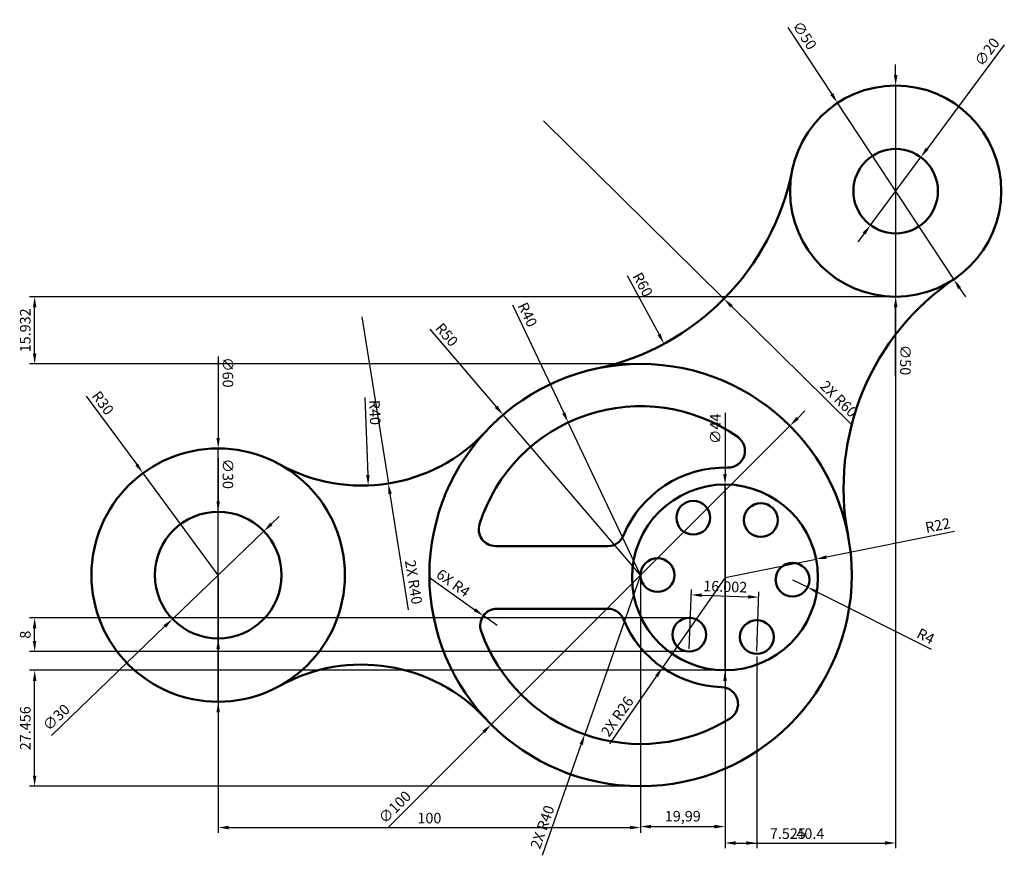
# Model space of a CAD drawing. Units: millimetres. Extents: x 2504 to 2737, y 1647 to 1845.
import ezdxf

# ---------------------------------------------------------------- set-up
doc = ezdxf.new("R2010")
doc.units = ezdxf.units.MM
doc.layers.add('M-DIMS', color=2, linetype='Continuous', lineweight=25)
doc.layers.add('M-OUTL', color=7, linetype='Continuous', lineweight=50)
doc.styles.get("Standard").update_dxf_attribs({"font": 'arial.ttf'})
doc.dimstyles.new('ISO-25', dxfattribs={"dimtxt": 2.5, "dimasz": 2.5, "dimexe": 1.25, "dimexo": 0.625, "dimtad": 1, "dimtxsty": 'Standard', "dimcen": 2.5, "dimadec": 0, "dimazin": 0, "dimtfac": 1, "dimtmove": 0, "dimatfit": 3, "dimfxl": 1, "dimarcsym": 0})

# ---------------------------------------------------------------- blocks, each defined once
blk = doc.blocks.new('*U1')
blk.add_circle((0, 0), 4)
blk = doc.blocks.new('*U2')
at = {"layer": 'M-OUTL', "color": 0, "linetype": 'ByBlock', "lineweight": -2, "transparency": 16777216}
for p, rotation in [((2663.06, 1727.21), 299.9999999999999), ((2679.05, 1726.66), 240), ((2686.57, 1712.54), 180), ((2662.11, 1699.51), 59.99999999999999), ((2678.11, 1698.96), 120)]:
    blk.add_blockref('*U1', p, dxfattribs=dict(at, rotation=rotation))
blk.add_blockref('*U1', (2654.59, 1713.63), dxfattribs=at)
blk = doc.blocks.new('*D3')
at = {"layer": 'Defpoints', "color": 0, "transparency": 16777216}
for p in [(2532.79, 1737.78), (2550.59, 1713.63)]:
    blk.add_point(p, dxfattribs=at)
at = {"layer": 'M-DIMS', "color": 0, "lineweight": -2, "transparency": 16777216}
for p, q in [((2519.37, 1755.97), (2531.3, 1739.79)), ((2550.59, 1713.63), (2532.79, 1737.78))]:
    blk.add_line(p, q, dxfattribs=at)
at = {"layer": 'M-DIMS', "color": 0, "transparency": 16777216}
blk.add_solid([(2531.64, 1740.03), (2530.97, 1739.54), (2532.79, 1737.78)], dxfattribs=at)
at = {"layer": 'M-DIMS', "color": 0, "transparency": 16777216, "insert": (2523.04, 1754.2), "char_height": 2.5, "attachment_point": 5, "rotation": 306.3975}
blk.add_mtext('R30', dxfattribs=at)
blk = doc.blocks.new('*D4')
at = {"layer": 'Defpoints', "color": 0, "transparency": 16777216}
for p in [(2584.59, 1774.82), (2586.11, 1734.85)]:
    blk.add_point(p, dxfattribs=at)
at = {"layer": 'M-DIMS', "color": 0, "lineweight": -2, "transparency": 16777216}
blk.add_line((2585.32, 1755.67), (2586.02, 1737.34), dxfattribs=at)
at = {"layer": 'M-DIMS', "color": 0, "transparency": 16777216}
blk.add_solid([(2586.44, 1737.36), (2585.6, 1737.33), (2586.11, 1734.85)], dxfattribs=at)
at = {"layer": 'M-DIMS', "color": 0, "transparency": 16777216, "insert": (2587.36, 1752.14), "char_height": 2.5, "attachment_point": 5, "rotation": 272.187}
blk.add_mtext('R40', dxfattribs=at)
blk = doc.blocks.new('*D5')
at = {"layer": 'Defpoints', "color": 0, "transparency": 16777216}
for p in [(2618.04, 1751.58), (2650.59, 1713.63)]:
    blk.add_point(p, dxfattribs=at)
at = {"layer": 'M-DIMS', "color": 0, "lineweight": -2, "transparency": 16777216}
for p, q in [((2600.66, 1771.84), (2616.41, 1753.48)), ((2650.59, 1713.63), (2618.04, 1751.58))]:
    blk.add_line(p, q, dxfattribs=at)
at = {"layer": 'M-DIMS', "color": 0, "transparency": 16777216}
blk.add_solid([(2616.73, 1753.75), (2616.09, 1753.21), (2618.04, 1751.58)], dxfattribs=at)
at = {"layer": 'M-DIMS', "color": 0, "transparency": 16777216, "insert": (2604.45, 1770.34), "char_height": 2.5, "attachment_point": 5, "rotation": 310.6195}
blk.add_mtext('R50', dxfattribs=at)
blk = doc.blocks.new('*D6')
at = {"layer": 'Defpoints', "color": 0, "transparency": 16777216}
for p in [(2633.46, 1749.78), (2650.59, 1713.63)]:
    blk.add_point(p, dxfattribs=at)
at = {"layer": 'M-DIMS', "color": 0, "lineweight": -2, "transparency": 16777216}
for p, q in [((2620.27, 1777.62), (2632.39, 1752.04)), ((2650.59, 1713.63), (2633.46, 1749.78))]:
    blk.add_line(p, q, dxfattribs=at)
at = {"layer": 'M-DIMS', "color": 0, "transparency": 16777216}
blk.add_solid([(2632.77, 1752.21), (2632.02, 1751.86), (2633.46, 1749.78)], dxfattribs=at)
at = {"layer": 'M-DIMS', "color": 0, "transparency": 16777216, "insert": (2623.54, 1775.17), "char_height": 2.5, "attachment_point": 5, "rotation": 295.3485}
blk.add_mtext('R40', dxfattribs=at)
blk = doc.blocks.new('*D7')
at = {"layer": 'Defpoints', "color": 0, "transparency": 16777216}
for p in [(2692.15, 1717.4), (2670.58, 1713.08)]:
    blk.add_point(p, dxfattribs=at)
at = {"layer": 'M-DIMS', "color": 0, "lineweight": -2, "transparency": 16777216}
for p, q in [((2724.9, 1723.96), (2694.6, 1717.9)), ((2670.58, 1713.08), (2692.15, 1717.4))]:
    blk.add_line(p, q, dxfattribs=at)
at = {"layer": 'M-DIMS', "color": 0, "transparency": 16777216}
blk.add_solid([(2694.52, 1718.3), (2694.69, 1717.49), (2692.15, 1717.4)], dxfattribs=at)
at = {"layer": 'M-DIMS', "color": 0, "transparency": 16777216, "insert": (2721, 1725.1), "char_height": 2.5, "attachment_point": 5, "rotation": 11.3281}
blk.add_mtext('R22', dxfattribs=at)
blk = doc.blocks.new('*D8')
at = {"layer": 'Defpoints', "color": 0, "transparency": 16777216}
for p in [(2686.57, 1712.54), (2690.15, 1710.74)]:
    blk.add_point(p, dxfattribs=at)
at = {"layer": 'M-DIMS', "color": 0, "lineweight": -2, "transparency": 16777216}
for p, q in [((2686.57, 1712.54), (2690.15, 1710.74)), ((2719.46, 1696.02), (2692.38, 1709.62))]:
    blk.add_line(p, q, dxfattribs=at)
at = {"layer": 'M-DIMS', "color": 0, "transparency": 16777216}
blk.add_solid([(2692.57, 1709.99), (2692.2, 1709.25), (2690.15, 1710.74)], dxfattribs=at)
at = {"layer": 'M-DIMS', "color": 0, "transparency": 16777216, "insert": (2717.95, 1698.88), "char_height": 2.5, "attachment_point": 5, "rotation": 333.3339}
blk.add_mtext('R4', dxfattribs=at)
blk = doc.blocks.new('*D9')
at = {"layer": 'Defpoints', "color": 0, "transparency": 16777216}
for p in [(2627.63, 1821.2), (2656.15, 1768.42)]:
    blk.add_point(p, dxfattribs=at)
at = {"layer": 'M-DIMS', "color": 0, "lineweight": -2, "transparency": 16777216}
blk.add_line((2647.43, 1784.55), (2654.96, 1770.62), dxfattribs=at)
at = {"layer": 'M-DIMS', "color": 0, "transparency": 16777216}
blk.add_solid([(2655.33, 1770.82), (2654.6, 1770.42), (2656.15, 1768.42)], dxfattribs=at)
at = {"layer": 'M-DIMS', "color": 0, "transparency": 16777216, "insert": (2650.82, 1782.28), "char_height": 2.5, "attachment_point": 5, "rotation": 298.3875}
blk.add_mtext('R60', dxfattribs=at)
blk = doc.blocks.new('*D10')
at = {"layer": 'Defpoints', "color": 0, "transparency": 16777216}
for p in [(2716.94, 1812.59), (2705.02, 1796.53)]:
    blk.add_point(p, dxfattribs=at)
at = {"layer": 'M-DIMS', "color": 0, "lineweight": -2, "transparency": 16777216}
for p, q in [((2736.7, 1839.2), (2718.43, 1814.6)), ((2705.02, 1796.53), (2716.94, 1812.59)), ((2703.53, 1794.52), (2702.04, 1792.52))]:
    blk.add_line(p, q, dxfattribs=at)
at = {"layer": 'M-DIMS', "color": 0, "transparency": 16777216}
for points in [[(2718.1, 1814.84), (2718.77, 1814.35), (2716.94, 1812.59)], [(2703.19, 1794.77), (2703.86, 1794.28), (2705.02, 1796.53)]]:
    blk.add_solid(points, dxfattribs=at)
at = {"layer": 'M-DIMS', "color": 0, "transparency": 16777216, "insert": (2732.87, 1837.34), "char_height": 2.5, "attachment_point": 5, "rotation": 53.4}
blk.add_mtext('∅20', dxfattribs=at)
blk = doc.blocks.new('*D11')
at = {"layer": 'Defpoints', "color": 0, "transparency": 16777216}
for p in [(2697.23, 1825.44), (2724.73, 1783.68)]:
    blk.add_point(p, dxfattribs=at)
at = {"layer": 'M-DIMS', "color": 0, "lineweight": -2, "transparency": 16777216}
for p, q in [((2685.45, 1843.33), (2695.85, 1827.53)), ((2724.73, 1783.68), (2697.23, 1825.44)), ((2726.11, 1781.59), (2727.48, 1779.51))]:
    blk.add_line(p, q, dxfattribs=at)
at = {"layer": 'M-DIMS', "color": 0, "transparency": 16777216}
for points in [[(2696.2, 1827.76), (2695.51, 1827.3), (2697.23, 1825.44)], [(2726.45, 1781.82), (2725.76, 1781.36), (2724.73, 1783.68)]]:
    blk.add_solid(points, dxfattribs=at)
at = {"layer": 'M-DIMS', "color": 0, "transparency": 16777216, "insert": (2689.17, 1841.26), "char_height": 2.5, "attachment_point": 5, "rotation": 303.3687}
blk.add_mtext('∅50', dxfattribs=at)
blk = doc.blocks.new('*D12')
at = {"layer": 'Defpoints', "color": 0, "transparency": 16777216}
for p in [(2561.4, 1724.02), (2539.78, 1703.23)]:
    blk.add_point(p, dxfattribs=at)
at = {"layer": 'M-DIMS', "color": 0, "lineweight": -2, "transparency": 16777216}
for p, q in [((2563.2, 1725.76), (2565, 1727.49)), ((2561.4, 1724.02), (2539.78, 1703.23)), ((2511.12, 1675.67), (2537.97, 1701.5))]:
    blk.add_line(p, q, dxfattribs=at)
at = {"layer": 'M-DIMS', "color": 0, "transparency": 16777216}
for points in [[(2562.91, 1726.06), (2563.49, 1725.46), (2561.4, 1724.02)], [(2537.69, 1701.8), (2538.26, 1701.2), (2539.78, 1703.23)]]:
    blk.add_solid(points, dxfattribs=at)
at = {"layer": 'M-DIMS', "color": 0, "transparency": 16777216, "insert": (2512.47, 1679.71), "char_height": 2.5, "attachment_point": 5, "rotation": 43.8787}
blk.add_mtext('∅30', dxfattribs=at)
blk = doc.blocks.new('*D13')
at = {"layer": 'Defpoints', "color": 0, "transparency": 16777216}
for p in [(2550.59, 1713.63), (2650.59, 1713.63), (2650.59, 1653.85)]:
    blk.add_point(p, dxfattribs=at)
at = {"layer": 'M-DIMS', "color": 0, "lineweight": -2, "transparency": 16777216}
for p, q in [((2550.59, 1713), (2550.59, 1652.6)), ((2650.59, 1713), (2650.59, 1652.6)), ((2553.09, 1653.85), (2648.09, 1653.85))]:
    blk.add_line(p, q, dxfattribs=at)
at = {"layer": 'M-DIMS', "color": 0, "transparency": 16777216}
for points in [[(2553.09, 1654.26), (2553.09, 1653.43), (2550.59, 1653.85)], [(2648.09, 1654.26), (2648.09, 1653.43), (2650.59, 1653.85)]]:
    blk.add_solid(points, dxfattribs=at)
at = {"layer": 'M-DIMS', "color": 0, "transparency": 16777216, "insert": (2600.59, 1655.75), "char_height": 2.5, "attachment_point": 5}
blk.add_mtext('100', dxfattribs=at)
blk = doc.blocks.new('*D14')
at = {"layer": 'Defpoints', "color": 0, "transparency": 16777216}
for p in [(2650.59, 1713.08), (2670.58, 1713.08), (2670.58, 1654.07)]:
    blk.add_point(p, dxfattribs=at)
at = {"layer": 'M-DIMS', "color": 0, "lineweight": -2, "transparency": 16777216}
for p, q in [((2650.59, 1712.46), (2650.59, 1652.82)), ((2670.58, 1712.46), (2670.58, 1652.82)), ((2653.09, 1654.07), (2668.08, 1654.07))]:
    blk.add_line(p, q, dxfattribs=at)
at = {"layer": 'M-DIMS', "color": 0, "transparency": 16777216}
for points in [[(2653.09, 1654.49), (2653.09, 1653.65), (2650.59, 1654.07)], [(2668.08, 1654.49), (2668.08, 1653.65), (2670.58, 1654.07)]]:
    blk.add_solid(points, dxfattribs=at)
at = {"layer": 'M-DIMS', "color": 0, "transparency": 16777216, "insert": (2660.58, 1656.2), "char_height": 2.5, "attachment_point": 5}
blk.add_mtext('19,99', dxfattribs=at)
blk = doc.blocks.new('*D15')
at = {"layer": 'Defpoints', "color": 0, "transparency": 16777216}
for p in [(2507.14, 1779.56), (2710.98, 1779.56), (2650.59, 1763.63)]:
    blk.add_point(p, dxfattribs=at)
at = {"layer": 'M-DIMS', "color": 0, "lineweight": -2, "transparency": 16777216}
for p, q in [((2710.35, 1779.56), (2505.89, 1779.56)), ((2507.14, 1766.13), (2507.14, 1777.06)), ((2649.96, 1763.63), (2505.89, 1763.63))]:
    blk.add_line(p, q, dxfattribs=at)
at = {"layer": 'M-DIMS', "color": 0, "transparency": 16777216}
for points in [[(2506.72, 1777.06), (2507.55, 1777.06), (2507.14, 1779.56)], [(2506.72, 1766.13), (2507.55, 1766.13), (2507.14, 1763.63)]]:
    blk.add_solid(points, dxfattribs=at)
at = {"layer": 'M-DIMS', "color": 0, "transparency": 16777216, "insert": (2505.24, 1771.59), "char_height": 2.5, "attachment_point": 5, "rotation": 90}
blk.add_mtext('15.932', dxfattribs=at)
blk = doc.blocks.new('*D16')
at = {"layer": 'Defpoints', "color": 0, "transparency": 16777216}
for p in [(2710.98, 1779.56), (2670.58, 1735.08), (2710.98, 1650.18)]:
    blk.add_point(p, dxfattribs=at)
at = {"layer": 'M-DIMS', "color": 0, "lineweight": -2, "transparency": 16777216}
for p, q in [((2710.98, 1778.93), (2710.98, 1648.93)), ((2670.58, 1734.46), (2670.58, 1648.93)), ((2673.08, 1650.18), (2708.48, 1650.18))]:
    blk.add_line(p, q, dxfattribs=at)
at = {"layer": 'M-DIMS', "color": 0, "transparency": 16777216}
for points in [[(2673.08, 1650.59), (2673.08, 1649.76), (2670.58, 1650.18)], [(2708.48, 1650.59), (2708.48, 1649.76), (2710.98, 1650.18)]]:
    blk.add_solid(points, dxfattribs=at)
at = {"layer": 'M-DIMS', "color": 0, "transparency": 16777216, "insert": (2690.78, 1652.08), "char_height": 2.5, "attachment_point": 5}
blk.add_mtext('40.4', dxfattribs=at)
blk = doc.blocks.new('*D17')
at = {"layer": 'Defpoints', "color": 0, "transparency": 16777216}
for p in [(2507.14, 1703.51), (2662.11, 1703.51), (2662.11, 1695.51)]:
    blk.add_point(p, dxfattribs=at)
at = {"layer": 'M-DIMS', "color": 0, "lineweight": -2, "transparency": 16777216}
for p, q in [((2661.49, 1703.51), (2505.89, 1703.51)), ((2507.14, 1698.01), (2507.14, 1701.01)), ((2661.49, 1695.51), (2505.89, 1695.51))]:
    blk.add_line(p, q, dxfattribs=at)
at = {"layer": 'M-DIMS', "color": 0, "transparency": 16777216}
for points in [[(2506.72, 1701.01), (2507.55, 1701.01), (2507.14, 1703.51)], [(2506.72, 1698.01), (2507.55, 1698.01), (2507.14, 1695.51)]]:
    blk.add_solid(points, dxfattribs=at)
at = {"layer": 'M-DIMS', "color": 0, "transparency": 16777216, "insert": (2505.24, 1699.51), "char_height": 2.5, "attachment_point": 5, "rotation": 90}
blk.add_mtext('8', dxfattribs=at)
blk = doc.blocks.new('*D18')
at = {"layer": 'Defpoints', "color": 0, "transparency": 16777216}
for p in [(2678.56, 1708.4), (2662.11, 1695.51), (2678.11, 1694.96)]:
    blk.add_point(p, dxfattribs=at)
at = {"layer": 'M-DIMS', "color": 0, "lineweight": -2, "transparency": 16777216}
for p, q in [((2662.13, 1696.13), (2662.61, 1710.2)), ((2665.07, 1708.86), (2676.06, 1708.49)), ((2678.13, 1695.59), (2678.61, 1709.65))]:
    blk.add_line(p, q, dxfattribs=at)
at = {"layer": 'M-DIMS', "color": 0, "transparency": 16777216}
for points in [[(2665.08, 1709.28), (2665.06, 1708.45), (2662.57, 1708.95)], [(2676.08, 1708.9), (2676.05, 1708.07), (2678.56, 1708.4)]]:
    blk.add_solid(points, dxfattribs=at)
at = {"layer": 'M-DIMS', "color": 0, "transparency": 16777216, "insert": (2670.63, 1710.58), "char_height": 2.5, "attachment_point": 5, "rotation": 358.0504}
blk.add_mtext('16.002', dxfattribs=at)
blk = doc.blocks.new('*D19')
at = {"layer": 'Defpoints', "color": 0, "transparency": 16777216}
for p in [(2507.14, 1691.08), (2670.58, 1691.08), (2650.59, 1663.63)]:
    blk.add_point(p, dxfattribs=at)
at = {"layer": 'M-DIMS', "color": 0, "lineweight": -2, "transparency": 16777216}
for p, q in [((2669.96, 1691.08), (2505.89, 1691.08)), ((2507.14, 1666.13), (2507.14, 1688.58)), ((2649.96, 1663.63), (2505.89, 1663.63))]:
    blk.add_line(p, q, dxfattribs=at)
at = {"layer": 'M-DIMS', "color": 0, "transparency": 16777216}
for points in [[(2506.72, 1688.58), (2507.55, 1688.58), (2507.14, 1691.08)], [(2506.72, 1666.13), (2507.55, 1666.13), (2507.14, 1663.63)]]:
    blk.add_solid(points, dxfattribs=at)
at = {"layer": 'M-DIMS', "color": 0, "transparency": 16777216, "insert": (2505.24, 1677.36), "char_height": 2.5, "attachment_point": 5, "rotation": 90}
blk.add_mtext('27.456', dxfattribs=at)
blk = doc.blocks.new('*D20')
at = {"layer": 'Defpoints', "color": 0, "transparency": 16777216}
for p in [(2678.11, 1694.96), (2670.58, 1691.08), (2678.11, 1650.18)]:
    blk.add_point(p, dxfattribs=at)
at = {"layer": 'M-DIMS', "color": 0, "lineweight": -2, "transparency": 16777216}
for p, q in [((2678.11, 1694.34), (2678.11, 1648.93)), ((2670.58, 1690.46), (2670.58, 1648.93)), ((2673.08, 1650.18), (2675.61, 1650.18)), ((2678.11, 1650.18), (2690.29, 1650.18))]:
    blk.add_line(p, q, dxfattribs=at)
at = {"layer": 'M-DIMS', "color": 0, "transparency": 16777216}
for points in [[(2673.08, 1650.59), (2673.08, 1649.76), (2670.58, 1650.18)], [(2675.61, 1650.59), (2675.61, 1649.76), (2678.11, 1650.18)]]:
    blk.add_solid(points, dxfattribs=at)
at = {"layer": 'M-DIMS', "color": 0, "transparency": 16777216, "insert": (2685.45, 1652.08), "char_height": 2.5, "attachment_point": 5}
blk.add_mtext('7.525', dxfattribs=at)
blk = doc.blocks.new('*D21')
at = {"layer": 'Defpoints', "color": 0, "transparency": 16777216}
for p in [(2550.59, 1743.63), (2550.59, 1683.63)]:
    blk.add_point(p, dxfattribs=at)
at = {"layer": 'M-DIMS', "color": 0, "lineweight": -2, "transparency": 16777216}
for p, q in [((2550.59, 1765.4), (2550.59, 1746.13)), ((2550.59, 1683.63), (2550.59, 1743.63)), ((2550.59, 1681.13), (2550.59, 1678.63))]:
    blk.add_line(p, q, dxfattribs=at)
at = {"layer": 'M-DIMS', "color": 0, "transparency": 16777216}
for points in [[(2551, 1746.13), (2550.17, 1746.13), (2550.59, 1743.63)], [(2551.01, 1681.13), (2550.17, 1681.13), (2550.59, 1683.63)]]:
    blk.add_solid(points, dxfattribs=at)
at = {"layer": 'M-DIMS', "color": 0, "transparency": 16777216, "insert": (2552.56, 1761.63), "char_height": 2.5, "attachment_point": 5, "rotation": 270.0006}
blk.add_mtext('∅60', dxfattribs=at)
blk = doc.blocks.new('*D22')
at = {"layer": 'Defpoints', "color": 0, "transparency": 16777216}
for p in [(2550.59, 1728.63), (2550.59, 1698.63)]:
    blk.add_point(p, dxfattribs=at)
at = {"layer": 'M-DIMS', "color": 0, "lineweight": -2, "transparency": 16777216}
for p, q in [((2550.59, 1741.4), (2550.59, 1731.13)), ((2550.59, 1698.63), (2550.59, 1728.63)), ((2550.59, 1696.13), (2550.59, 1693.63))]:
    blk.add_line(p, q, dxfattribs=at)
at = {"layer": 'M-DIMS', "color": 0, "transparency": 16777216}
for points in [[(2551, 1731.13), (2550.17, 1731.13), (2550.59, 1728.63)], [(2551.01, 1696.13), (2550.17, 1696.13), (2550.59, 1698.63)]]:
    blk.add_solid(points, dxfattribs=at)
at = {"layer": 'M-DIMS', "color": 0, "transparency": 16777216, "insert": (2552.56, 1737.63), "char_height": 2.5, "attachment_point": 5, "rotation": 270.0012}
blk.add_mtext('∅30', dxfattribs=at)
blk = doc.blocks.new('*D23')
at = {"layer": 'Defpoints', "color": 0, "transparency": 16777216}
for p in [(2685.94, 1748.98), (2615.23, 1678.27)]:
    blk.add_point(p, dxfattribs=at)
at = {"layer": 'M-DIMS', "color": 0, "lineweight": -2, "transparency": 16777216}
for p, q in [((2687.71, 1750.75), (2689.48, 1752.52)), ((2685.94, 1748.98), (2615.23, 1678.27)), ((2590.67, 1653.71), (2613.46, 1676.5))]:
    blk.add_line(p, q, dxfattribs=at)
at = {"layer": 'M-DIMS', "color": 0, "transparency": 16777216}
for points in [[(2687.42, 1751.05), (2688.01, 1750.46), (2685.94, 1748.98)], [(2613.17, 1676.8), (2613.76, 1676.21), (2615.23, 1678.27)]]:
    blk.add_solid(points, dxfattribs=at)
at = {"layer": 'M-DIMS', "color": 0, "transparency": 16777216, "insert": (2592.63, 1658.45), "char_height": 2.5, "attachment_point": 5, "rotation": 44.9996}
blk.add_mtext('∅100', dxfattribs=at)
blk = doc.blocks.new('*D24')
at = {"layer": 'Defpoints', "color": 0, "transparency": 16777216}
for p in [(2710.98, 1829.56), (2710.98, 1779.56)]:
    blk.add_point(p, dxfattribs=at)
at = {"layer": 'M-DIMS', "color": 0, "lineweight": -2, "transparency": 16777216}
for p, q in [((2710.98, 1832.06), (2710.98, 1834.56)), ((2710.98, 1829.56), (2710.98, 1779.56)), ((2710.98, 1760.79), (2710.98, 1777.06))]:
    blk.add_line(p, q, dxfattribs=at)
at = {"layer": 'M-DIMS', "color": 0, "transparency": 16777216}
for points in [[(2711.4, 1832.06), (2710.56, 1832.06), (2710.98, 1829.56)], [(2711.4, 1777.06), (2710.56, 1777.06), (2710.98, 1779.56)]]:
    blk.add_solid(points, dxfattribs=at)
at = {"layer": 'M-DIMS', "color": 0, "transparency": 16777216, "insert": (2712.95, 1764.56), "char_height": 2.5, "attachment_point": 5, "rotation": 270.0005}
blk.add_mtext('∅50', dxfattribs=at)
blk = doc.blocks.new('*D25')
at = {"layer": 'Defpoints', "color": 0, "transparency": 16777216}
for p in [(2584.59, 1774.82), (2590.88, 1735.31)]:
    blk.add_point(p, dxfattribs=at)
at = {"layer": 'M-DIMS', "color": 0, "lineweight": -2, "transparency": 16777216}
for p, q in [((2584.59, 1774.82), (2590.88, 1735.31)), ((2595.65, 1705.38), (2591.28, 1732.85))]:
    blk.add_line(p, q, dxfattribs=at)
at = {"layer": 'M-DIMS', "color": 0, "transparency": 16777216}
blk.add_solid([(2591.69, 1732.91), (2590.86, 1732.78), (2590.88, 1735.31)], dxfattribs=at)
at = {"layer": 'M-DIMS', "color": 0, "transparency": 16777216, "insert": (2596.54, 1711.91), "char_height": 2.5, "attachment_point": 5, "rotation": 279.054}
blk.add_mtext('2X R40', dxfattribs=at)
blk = doc.blocks.new('*D26')
at = {"layer": 'Defpoints', "color": 0, "transparency": 16777216}
for p in [(2650.59, 1713.63), (2637.37, 1675.88)]:
    blk.add_point(p, dxfattribs=at)
at = {"layer": 'M-DIMS', "color": 0, "lineweight": -2, "transparency": 16777216}
for p, q in [((2650.59, 1713.63), (2637.37, 1675.88)), ((2627.35, 1647.27), (2636.54, 1673.52))]:
    blk.add_line(p, q, dxfattribs=at)
at = {"layer": 'M-DIMS', "color": 0, "transparency": 16777216}
blk.add_solid([(2636.15, 1673.65), (2636.93, 1673.38), (2637.37, 1675.88)], dxfattribs=at)
at = {"layer": 'M-DIMS', "color": 0, "transparency": 16777216, "insert": (2627.64, 1653.85), "char_height": 2.5, "attachment_point": 5, "rotation": 70.6989}
blk.add_mtext('2X R40', dxfattribs=at)
blk = doc.blocks.new('*D27')
at = {"layer": 'Defpoints', "color": 0, "transparency": 16777216}
for p in [(2670.58, 1713.08), (2655.78, 1691.71)]:
    blk.add_point(p, dxfattribs=at)
at = {"layer": 'M-DIMS', "color": 0, "lineweight": -2, "transparency": 16777216}
for p, q in [((2670.58, 1713.08), (2655.78, 1691.71)), ((2643.31, 1673.68), (2654.36, 1689.65))]:
    blk.add_line(p, q, dxfattribs=at)
at = {"layer": 'M-DIMS', "color": 0, "transparency": 16777216}
blk.add_solid([(2654.02, 1689.89), (2654.7, 1689.41), (2655.78, 1691.71)], dxfattribs=at)
at = {"layer": 'M-DIMS', "color": 0, "transparency": 16777216, "insert": (2645.34, 1679.96), "char_height": 2.5, "attachment_point": 5, "rotation": 55.3063}
blk.add_mtext('2X R26', dxfattribs=at)
blk = doc.blocks.new('*D28')
at = {"layer": 'Defpoints', "color": 0, "transparency": 16777216}
for p in [(2613.37, 1703.98), (2616.63, 1701.67)]:
    blk.add_point(p, dxfattribs=at)
at = {"layer": 'M-DIMS', "color": 0, "lineweight": -2, "transparency": 16777216}
for p, q in [((2600.59, 1713.03), (2611.33, 1705.43)), ((2616.63, 1701.67), (2613.37, 1703.98))]:
    blk.add_line(p, q, dxfattribs=at)
at = {"layer": 'M-DIMS', "color": 0, "transparency": 16777216}
blk.add_solid([(2611.57, 1705.77), (2611.09, 1705.09), (2613.37, 1703.98)], dxfattribs=at)
at = {"layer": 'M-DIMS', "color": 0, "transparency": 16777216, "insert": (2606.04, 1711.5), "char_height": 2.5, "attachment_point": 5, "rotation": 324.6997}
blk.add_mtext('6X R4', dxfattribs=at)
blk = doc.blocks.new('*D29')
at = {"layer": 'Defpoints', "color": 0, "transparency": 16777216}
for p in [(2627.63, 1821.2), (2670.33, 1779.06)]:
    blk.add_point(p, dxfattribs=at)
at = {"layer": 'M-DIMS', "color": 0, "lineweight": -2, "transparency": 16777216}
for p, q in [((2627.63, 1821.2), (2670.33, 1779.06)), ((2700.45, 1749.34), (2672.11, 1777.3))]:
    blk.add_line(p, q, dxfattribs=at)
at = {"layer": 'M-DIMS', "color": 0, "transparency": 16777216}
blk.add_solid([(2672.4, 1777.6), (2671.82, 1777.01), (2670.33, 1779.06)], dxfattribs=at)
at = {"layer": 'M-DIMS', "color": 0, "transparency": 16777216, "insert": (2697.29, 1755.13), "char_height": 2.5, "attachment_point": 5, "rotation": 315.3784}
blk.add_mtext('2X R60', dxfattribs=at)
blk = doc.blocks.new('*D30')
at = {"layer": 'Defpoints', "color": 0, "transparency": 16777216}
for p in [(2670.58, 1735.08), (2670.58, 1691.08)]:
    blk.add_point(p, dxfattribs=at)
at = {"layer": 'M-DIMS', "color": 0, "lineweight": -2, "transparency": 16777216}
for p, q in [((2670.58, 1752.05), (2670.58, 1737.58)), ((2670.58, 1691.08), (2670.58, 1735.08)), ((2670.58, 1688.58), (2670.58, 1686.08))]:
    blk.add_line(p, q, dxfattribs=at)
at = {"layer": 'M-DIMS', "color": 0, "transparency": 16777216}
for points in [[(2670.16, 1737.58), (2671, 1737.58), (2670.58, 1735.08)], [(2670.16, 1688.58), (2671, 1688.58), (2670.58, 1691.08)]]:
    blk.add_solid(points, dxfattribs=at)
at = {"layer": 'M-DIMS', "color": 0, "transparency": 16777216, "insert": (2668.61, 1748.28), "char_height": 2.5, "attachment_point": 5, "rotation": 89.9997}
blk.add_mtext('∅44', dxfattribs=at)

msp = doc.modelspace()

# ---------------------------------------------------------------- linework, layer by layer
at = {"layer": 'M-OUTL'}
for p, q in [((2642.837, 1720.4971), (2616.2684, 1720.4971)), ((2642.837, 1705.6696), (2616.6324, 1705.6696))]:
    msp.add_line(p, q, dxfattribs=at)
for centre, radius in [((2710.9798, 1804.5598), 25), ((2710.9798, 1804.5598), 10), ((2650.5883, 1713.6278), 50), ((2550.5883, 1713.6278), 30), ((2670.5809, 1713.0834), 22), ((2550.5883, 1713.6278), 15)]:
    msp.add_circle(centre, radius, dxfattribs=at)
for centre, radius, start, end in [((2627.6253, 1821.2043), 60, 282.049362, 348.707517), ((2758.6502, 1734.1856), 60, 124.113141, 190.771295), ((2650.5883, 1713.6278), 40, 54.882444, 162.426663), ((2584.5883, 1774.816), 40, 240.940719, 317.166572), ((2671.2975, 1743.0748), 4, 268.63122, 54.882444), ((2670.5809, 1713.0834), 26, 88.63122, 157.637945), ((2616.2684, 1724.4971), 4, 162.426663, 270), ((2642.837, 1724.4971), 4, 270, 337.637945), ((2650.5883, 1713.6278), 40, 358.093678, 358.440234), ((2616.6324, 1701.6696), 4, 90, 199.400562), ((2642.837, 1701.6696), 4, 22.362055, 90), ((2670.5809, 1713.0834), 26, 202.362055, 268.249248), ((2650.5883, 1713.6278), 40, 199.400562, 301.998024), ((2584.5883, 1652.4395), 40, 42.833428, 119.059281), ((2669.6644, 1683.0974), 4, 301.998024, 88.249248)]:
    msp.add_arc(centre, radius, start, end, dxfattribs=at)

# ---------------------------------------------------------------- block references
msp.add_blockref('*U2', (0, 0), dxfattribs=at)

# ---------------------------------------------------------------- dimensions: what is measured, and where the dimension line sits
at = {"layer": 'M-DIMS'}
for p1, p2, override, picture, middle in [((2724.7304, 1783.6811), (2697.2291, 1825.4385), {"dimclrd": 0, "dimclre": 0, "dimclrt": 0}, '*D11', (2687.5234, 1840.1756)), ((2705.0175, 1796.5316), (2716.942, 1812.588), {"dimclrd": 0, "dimclre": 0, "dimclrt": 0}, '*D10', (2734.4544, 1836.1685)), ((2710.9795, 1829.5598), (2710.98, 1779.5598), {"dimdec": 0, "dimlfac": 1, "dimrnd": 0, "dimzin": 0, "dimdsep": 46, "dimlunit": 2}, '*D24', (2710.9801, 1764.5598)), ((2550.5886, 1683.6278), (2550.588, 1743.6278), {"dimdec": 0, "dimlfac": 1, "dimrnd": 0, "dimzin": 0, "dimdsep": 46, "dimlunit": 2}, '*D21', (2550.5878, 1761.6278)), ((2685.9439, 1748.9828), (2615.2327, 1678.2727), {"dimdec": 0, "dimlfac": 1, "dimrnd": 0, "dimzin": 0, "dimdsep": 46, "dimlunit": 2}, '*D23', (2594.0193, 1657.0597)), ((2670.5808, 1691.0834), (2670.581, 1735.0834), {"dimdec": 0, "dimlfac": 1, "dimrnd": 0, "dimzin": 0, "dimdsep": 46, "dimlunit": 2}, '*D30', (2670.5811, 1748.2834)), ((2550.5886, 1698.6278), (2550.588, 1728.6278), {"dimdec": 0, "dimlfac": 1, "dimrnd": 0, "dimzin": 0, "dimdsep": 46, "dimlunit": 2}, '*D22', (2550.5878, 1737.6278)), ((2561.4004, 1724.0248), (2539.7762, 1703.2308), {"dimclrd": 0, "dimclre": 0, "dimclrt": 0}, '*D12', (2513.8381, 1678.2886))]:
    dim = msp.add_diameter_dim_2p(p1=p1, p2=p2, dimstyle='ISO-25', override=override, dxfattribs=at)
    dim.commit()
    dim.dimension.update_dxf_attribs({"geometry": picture, "text_midpoint": middle, "dimtype": 163})
for center, mpoint, picture, middle in [((2627.6253, 1821.2043), (2656.1513, 1768.4191), '*D9', (2649.15, 1781.3744)), ((2650.5883, 1713.6278), (2633.4634, 1749.7766), '*D6', (2621.8173, 1774.3603)), ((2584.5883, 1774.816), (2586.1148, 1734.8451), '*D4', (2585.4571, 1752.0656)), ((2650.5883, 1713.6278), (2618.0367, 1751.5803), '*D5', (2603.0103, 1769.0998)), ((2550.5883, 1713.6278), (2532.7868, 1737.7754), '*D3', (2521.5134, 1753.0676)), ((2670.5809, 1713.0834), (2692.1523, 1717.4048), '*D7', (2721.3688, 1723.2577)), ((2686.5735, 1712.539), (2690.148, 1710.7438), '*D8', (2717.1059, 1697.2054))]:
    dim = msp.add_radius_dim(center=center, mpoint=mpoint, dimstyle='ISO-25', override={"dimclrd": 0, "dimclre": 0, "dimclrt": 0}, dxfattribs=at)
    dim.commit()
    dim.dimension.update_dxf_attribs({"geometry": picture, "text_midpoint": middle, "dimtype": 164})
for center, mpoint, picture, middle in [((2627.6253, 1821.2043), (2670.331, 1779.059), '*D29', (2695.9544, 1753.7718)), ((2584.5883, 1774.816), (2590.8829, 1735.3144), '*D25', (2594.6597, 1711.6134)), ((2650.5883, 1713.6278), (2637.367, 1675.876), '*D26', (2629.4342, 1653.2249)), ((2670.5809, 1713.0834), (2655.782, 1691.706), '*D27', (2646.9027, 1678.8796))]:
    dim = msp.add_radius_dim(center=center, mpoint=mpoint, text='2X <>', dimstyle='ISO-25', override={"dimdec": 0, "dimlfac": 1, "dimrnd": 0, "dimzin": 0, "dimdsep": 46, "dimlunit": 2}, dxfattribs=at)
    dim.commit()
    dim.dimension.update_dxf_attribs({"geometry": picture, "text_midpoint": middle, "dimtype": 164})
for base, p1, p2, angle, override, picture, middle in [((2507.1383, 1779.5598), (2650.5883, 1763.6278), (2710.9798, 1779.5598), 90, {"dimdec": 3, "dimlfac": 1, "dimrnd": 0, "dimzin": 0, "dimdsep": 46, "dimlunit": 2}, '*D15', (2505.236, 1771.5938)), ((2678.5633, 1708.4034), (2662.1131, 1695.5056), (2678.1057, 1694.9612), 358.050383, {"dimdec": 3, "dimlfac": 1, "dimrnd": 0, "dimzin": 0, "dimdsep": 46, "dimlunit": 2}, '*D18', (2670.6317, 1710.5759)), ((2507.1383, 1703.5056), (2662.1131, 1695.5056), (2662.1131, 1703.5056), 90, {"dimdec": 0, "dimlfac": 1, "dimrnd": 0, "dimzin": 0, "dimdsep": 46, "dimlunit": 2}, '*D17', (2505.2369, 1699.5056)), ((2507.1383, 1691.0834), (2650.5883, 1663.6278), (2670.5809, 1691.0834), 90, {"dimdec": 3, "dimlfac": 1, "dimrnd": 0, "dimzin": 0, "dimdsep": 46, "dimlunit": 2}, '*D19', (2505.2369, 1677.3556))]:
    dim = msp.add_linear_dim(base=base, p1=p1, p2=p2, angle=angle, dimstyle='ISO-25', override=override, dxfattribs=at)
    dim.commit()
    dim.dimension.update_dxf_attribs({"geometry": picture, "text_midpoint": middle})
for base, p1, p2, override, picture, middle in [((2710.9798, 1650.1778), (2670.5809, 1735.0834), (2710.9798, 1779.5598), {"dimdec": 1, "dimlfac": 1, "dimrnd": 0, "dimzin": 0, "dimdsep": 46, "dimlunit": 2}, '*D16', (2690.7803, 1652.0792)), ((2650.5883, 1653.8452), (2550.5883, 1713.6278), (2650.5883, 1713.6278), {"dimclrd": 0, "dimclre": 0, "dimclrt": 0}, '*D13', (2600.5883, 1655.7467)), ((2670.5809, 1654.07), (2650.5883, 1713.0834), (2670.5809, 1713.0834), {"dimclrd": 0, "dimclre": 0, "dimclrt": 0}, '*D14', (2660.5846, 1656.1974)), ((2678.1057, 1650.1778), (2670.5809, 1691.0834), (2678.1057, 1694.9612), {"dimdec": 3, "dimlfac": 1, "dimrnd": 0, "dimzin": 0, "dimdsep": 46, "dimlunit": 2}, '*D20', (2685.448, 1652.0792))]:
    dim = msp.add_linear_dim(base=base, p1=p1, p2=p2, dimstyle='ISO-25', override=override, dxfattribs=at)
    dim.commit()
    dim.dimension.update_dxf_attribs({"geometry": picture, "text_midpoint": middle})
dim = msp.add_radius_dim(center=(2616.6324, 1701.6696), mpoint=(2613.3679, 1703.9811), text='6X <>', dimstyle='ISO-25', override={"dimdec": 0, "dimlfac": 1, "dimrnd": 0, "dimzin": 0, "dimdsep": 46, "dimlunit": 2}, dxfattribs=at)
dim.commit()
dim.dimension.update_dxf_attribs({"geometry": '*D28', "text_midpoint": (2606.0374, 1711.5012)})

doc.saveas('drawing.dxf')
